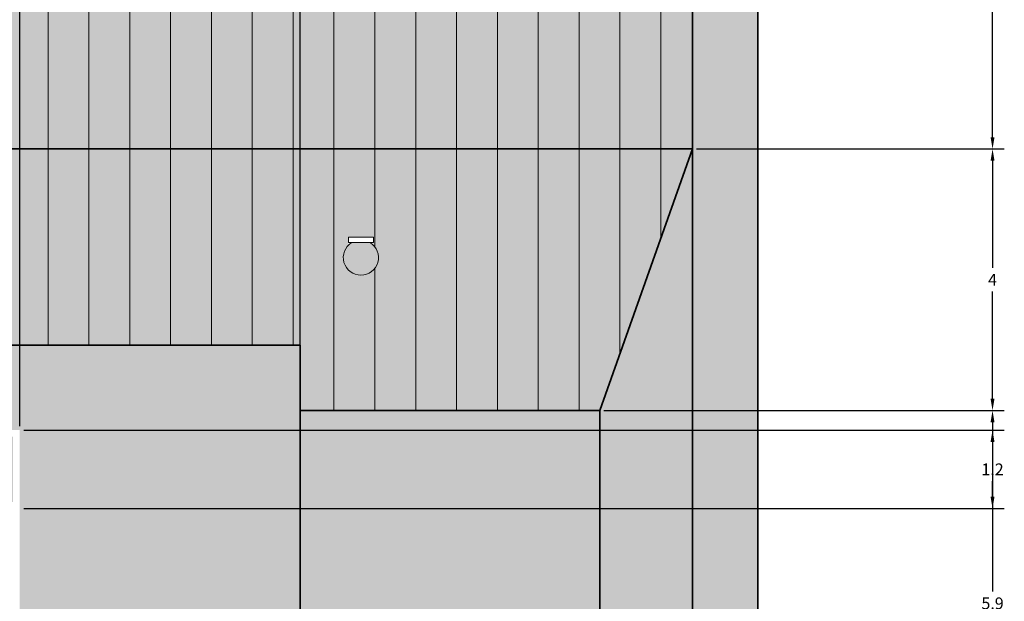
# Model space of a CAD drawing. Units: inches. Extents: x 18 to 59.8, y 2.7 to 81.2.
# Tile 9 of 9: x 44.6 to 59.6, y 54.5 to 63.4. Entities that reach past the tile are written whole.
import ezdxf

# ---------------------------------------------------------------- set-up
doc = ezdxf.new("R2010")
doc.units = ezdxf.units.IN
doc.header["$MEASUREMENT"] = 0
for name, color, linetype, lineweight in [('A-ANNO-DIMS', 2, 'Continuous', 18), ('A-ELEV', 7, 'Continuous', 35), ('A-ELEV-PATT', 8, 'Continuous', 13), ('E-LITE', 2, 'Continuous', 18)]:
    doc.layers.add(name, color=color, linetype=linetype, lineweight=lineweight)
doc.styles.get("Standard").update_dxf_attribs({"font": 'arial.ttf'})
doc.dimstyles.get("Standard").update_dxf_attribs({"dimtxt": 0.18, "dimasz": 0.18, "dimexe": 0.18, "dimexo": 0.0625, "dimgap": 0.09, "dimtad": 0, "dimtih": 1, "dimtoh": 1, "dimdec": 1, "dimzin": 0, "dimdsep": 46, "dimlunit": 3, "dimtxsty": 'Standard', "dimcen": 0.09, "dimadec": 0, "dimazin": 0, "dimtfac": 1, "dimtdec": 1, "dimtofl": 0, "dimtmove": 0, "dimatfit": 3, "dimfxl": 1, "dimtolj": 1, "dimtzin": 0, "dimarcsym": 0})

# ---------------------------------------------------------------- blocks, each defined once
blk = doc.blocks.new('LIGHT-CEILING-SPOT')
blk.add_lwpolyline([(0.0786613461026633, 0.4966935902599801), (0.4594351322230353, 0.4966935902599801), (0.4594351322230353, 0.5789100459995425), (0.0786613461026633, 0.5789100459995425)], close=True)
blk.add_arc((0.2690482391628493, 0.2688350374553394), 0.2689667806744183, 122.0956315451972, 57.90436845480281)
blk = doc.blocks.new('*D19')
at = {"layer": 'A-ANNO-DIMS', "color": 0, "lineweight": -2, "transparency": 16777216}
for p, q in [((53.50256100000002, 57.44074800000003), (59.62997100000006, 57.44074800000003)), ((59.44997100000005, 57.26074800000002), (59.44997100000005, 54.67265113778992)), ((59.44997100000005, 51.72074800000003), (59.44997100000005, 54.30884486221012)), ((53.42247100000003, 51.54074800000003), (59.62997100000006, 51.54074800000003))]:
    blk.add_line(p, q, dxfattribs=at)
at = {"layer": 'A-ANNO-DIMS', "color": 0, "transparency": 16777216}
for points in [[(59.41997100000005, 57.26074800000002), (59.47997100000005, 57.26074800000002), (59.44997100000005, 57.44074800000003)], [(59.41997100000005, 51.72074800000003), (59.47997100000005, 51.72074800000003), (59.44997100000005, 51.54074800000003)]]:
    blk.add_solid(points, dxfattribs=at)
at = {"layer": 'Defpoints', "color": 0, "transparency": 16777216}
for p in [(53.44006100000003, 57.44074800000003), (59.44997100000005, 57.44074800000003), (53.35997100000003, 51.54074800000003)]:
    blk.add_point(p, dxfattribs=at)
at = {"layer": 'A-ANNO-DIMS', "color": 0, "transparency": 16777216, "insert": (59.44997100000005, 54.49074799999999), "char_height": 0.18, "attachment_point": 5}
blk.add_mtext('\\A1;5.9', dxfattribs=at)
blk = doc.blocks.new('*D20')
at = {"layer": 'A-ANNO-DIMS', "color": 0, "lineweight": -2, "transparency": 16777216}
for p, q in [((54.92247100000003, 61.44074800000002), (59.62997100000006, 61.44074800000002)), ((59.44997100000005, 61.26074800000003), (59.44997100000005, 59.62074800000003)), ((59.44997100000005, 57.62074800000003), (59.44997100000005, 59.26074800000002)), ((53.50256100000002, 57.44074800000003), (59.62997100000006, 57.44074800000003))]:
    blk.add_line(p, q, dxfattribs=at)
at = {"layer": 'A-ANNO-DIMS', "color": 0, "transparency": 16777216}
for points in [[(59.41997100000005, 61.26074800000003), (59.47997100000005, 61.26074800000003), (59.44997100000005, 61.44074800000002)], [(59.41997100000005, 57.62074800000003), (59.47997100000005, 57.62074800000003), (59.44997100000005, 57.44074800000003)]]:
    blk.add_solid(points, dxfattribs=at)
at = {"layer": 'Defpoints', "color": 0, "transparency": 16777216}
for p in [(54.85997100000003, 61.44074800000002), (59.44997100000005, 61.44074800000002), (53.44006100000003, 57.44074800000003)]:
    blk.add_point(p, dxfattribs=at)
at = {"layer": 'A-ANNO-DIMS', "color": 0, "transparency": 16777216, "insert": (59.44997100000006, 59.44074799999999), "char_height": 0.18, "attachment_point": 5}
blk.add_mtext('\\A1;4', dxfattribs=at)
blk = doc.blocks.new('*D21')
at = {"layer": 'A-ANNO-DIMS', "color": 0, "lineweight": -2, "transparency": 16777216}
for p, q in [((54.92247100000003, 69.44074800000001), (59.62997100000006, 69.44074800000001)), ((59.44997100000005, 69.26074800000002), (59.44997100000005, 65.62265113778993)), ((59.44997100000005, 61.62074800000002), (59.44997100000005, 65.25884486221013)), ((54.92247100000003, 61.44074800000002), (59.62997100000006, 61.44074800000002))]:
    blk.add_line(p, q, dxfattribs=at)
at = {"layer": 'A-ANNO-DIMS', "color": 0, "transparency": 16777216}
for points in [[(59.41997100000005, 69.26074800000002), (59.47997100000005, 69.26074800000002), (59.44997100000005, 69.44074800000001)], [(59.41997100000005, 61.62074800000002), (59.47997100000005, 61.62074800000002), (59.44997100000005, 61.44074800000002)]]:
    blk.add_solid(points, dxfattribs=at)
at = {"layer": 'Defpoints', "color": 0, "transparency": 16777216}
for p in [(54.85997100000003, 69.44074800000001), (59.44997100000005, 69.44074800000001), (54.85997100000003, 61.44074800000002)]:
    blk.add_point(p, dxfattribs=at)
at = {"layer": 'A-ANNO-DIMS', "color": 0, "transparency": 16777216, "insert": (59.44997100000006, 65.440748), "char_height": 0.18, "attachment_point": 5}
blk.add_mtext('\\A1;8', dxfattribs=at)
blk = doc.blocks.new('*D51')
at = {"layer": 'A-ANNO-DIMS', "color": 0, "lineweight": -2, "transparency": 16777216}
for p, q in [((34.011642, 44.50324799999999), (34.011642, 81.210748)), ((48.859971, 43.503248), (48.859971, 81.210748)), ((34.191642, 81.03074799999999), (40.98046543587994, 81.03074799999999)), ((48.679971, 81.03074799999999), (41.89114756412005, 81.03074799999999))]:
    blk.add_line(p, q, dxfattribs=at)
at = {"layer": 'A-ANNO-DIMS', "color": 0, "transparency": 16777216}
for points in [[(34.191642, 81.060748), (34.191642, 81.00074799999999), (34.011642, 81.03074799999999)], [(48.679971, 81.060748), (48.679971, 81.00074799999999), (48.859971, 81.03074799999999)]]:
    blk.add_solid(points, dxfattribs=at)
at = {"layer": 'Defpoints', "color": 0, "transparency": 16777216}
for p in [(48.859971, 81.03074799999999), (34.011642, 44.440748), (48.859971, 43.440748)]:
    blk.add_point(p, dxfattribs=at)
at = {"layer": 'A-ANNO-DIMS', "color": 0, "transparency": 16777216, "insert": (41.43580649999999, 81.03074799999999), "char_height": 0.18, "attachment_point": 5}
blk.add_mtext('\\A1;14.848', dxfattribs=at)
blk = doc.blocks.new('*D62')
at = {"layer": 'A-ANNO-DIMS', "color": 0, "lineweight": -2, "transparency": 16777216}
for p, q in [((32.567078, 57.203248), (32.567078, 81.210748)), ((44.567078, 57.203248), (44.567078, 81.210748)), ((32.747078, 81.03074799999999), (38.35754866848568, 81.03074799999999)), ((44.387078, 81.03074799999999), (38.77660733151433, 81.03074799999999))]:
    blk.add_line(p, q, dxfattribs=at)
at = {"layer": 'A-ANNO-DIMS', "color": 0, "transparency": 16777216}
for points in [[(32.747078, 81.060748), (32.747078, 81.00074799999999), (32.567078, 81.03074799999999)], [(44.387078, 81.060748), (44.387078, 81.00074799999999), (44.567078, 81.03074799999999)]]:
    blk.add_solid(points, dxfattribs=at)
at = {"layer": 'Defpoints', "color": 0, "transparency": 16777216}
for p in [(44.567078, 81.03074799999999), (32.567078, 57.140748), (44.567078, 57.140748)]:
    blk.add_point(p, dxfattribs=at)
at = {"layer": 'A-ANNO-DIMS', "color": 0, "transparency": 16777216, "insert": (38.567078, 81.03074799999999), "char_height": 0.18, "attachment_point": 5}
blk.add_mtext('\\A1;12', dxfattribs=at)
blk = doc.blocks.new('*D63')
at = {"layer": 'A-ANNO-DIMS', "color": 0, "lineweight": -2, "transparency": 16777216}
for p, q in [((44.567078, 57.203248), (44.567078, 81.210748)), ((48.859971, 58.503248), (48.859971, 81.210748)), ((44.747078, 81.03074799999999), (46.31619844270123, 81.03074799999999)), ((48.679971, 81.03074799999999), (47.11085055729877, 81.03074799999999))]:
    blk.add_line(p, q, dxfattribs=at)
at = {"layer": 'A-ANNO-DIMS', "color": 0, "transparency": 16777216}
for points in [[(44.747078, 81.060748), (44.747078, 81.00074799999999), (44.567078, 81.03074799999999)], [(48.679971, 81.060748), (48.679971, 81.00074799999999), (48.859971, 81.03074799999999)]]:
    blk.add_solid(points, dxfattribs=at)
at = {"layer": 'Defpoints', "color": 0, "transparency": 16777216}
for p in [(48.859971, 81.03074799999999), (48.859971, 58.440748), (44.567078, 57.140748)]:
    blk.add_point(p, dxfattribs=at)
at = {"layer": 'A-ANNO-DIMS', "color": 0, "transparency": 16777216, "insert": (46.7135245, 81.03074799999999), "char_height": 0.18, "attachment_point": 5}
blk.add_mtext('\\A1;4.293', dxfattribs=at)
blk = doc.blocks.new('*D64')
at = {"layer": 'A-ANNO-DIMS', "color": 0, "lineweight": -2, "transparency": 16777216}
for p, q in [((44.62957800000001, 57.14074800000003), (59.62997100000006, 57.14074800000004)), ((59.44997100000005, 56.96074800000004), (59.44997100000005, 56.7211163492497)), ((59.44997100000005, 56.12074800000003), (59.44997100000005, 56.36037965075037)), ((44.62957800000001, 55.94074800000003), (59.62997100000006, 55.94074800000004))]:
    blk.add_line(p, q, dxfattribs=at)
at = {"layer": 'A-ANNO-DIMS', "color": 0, "transparency": 16777216}
for points in [[(59.41997100000005, 56.96074800000004), (59.47997100000005, 56.96074800000004), (59.44997100000005, 57.14074800000004)], [(59.41997100000005, 56.12074800000003), (59.47997100000005, 56.12074800000003), (59.44997100000005, 55.94074800000004)]]:
    blk.add_solid(points, dxfattribs=at)
at = {"layer": 'Defpoints', "color": 0, "transparency": 16777216}
for p in [(44.56707800000001, 57.14074800000003), (59.44997100000005, 57.14074800000004), (44.56707800000001, 55.94074800000003)]:
    blk.add_point(p, dxfattribs=at)
at = {"layer": 'A-ANNO-DIMS', "color": 0, "transparency": 16777216, "insert": (59.44997100000005, 56.540748), "char_height": 0.18, "attachment_point": 5}
blk.add_mtext('\\A1;1.2', dxfattribs=at)

msp = doc.modelspace()

# ---------------------------------------------------------------- hatches: boundary and pattern name
at = {"layer": 'A-ELEV-PATT'}
h = msp.add_hatch(color=256, dxfattribs=at)
h.set_gradient(color1=(255, 255, 255), color2=(199, 200, 202))
h.paths.add_polyline_path([(38.85997087182833, 75.45212783007513, 0.4125526599533602), (36.85997087192615, 77.44074750583997), (21.85997087182832, 77.44074750583995), (21.85997087182832, 22.44074750583995), (22.85997087182833, 22.44074750583995), (48.85997087182833, 22.44074750583996), (48.85997087182833, 30.92342676155402, 0.4074472928332927), (48.33023903111634, 31.44074750583995), (30.40609029701442, 31.44074750583996, -0.7603989452129261), (34.01164157247843, 44.44074750583996), (47.85997087182832, 44.44074750583995, -0.4142135623730951), (48.85997087182833, 43.44074750583994), (48.85997087182833, 48.44074750583995, 0.4142135623730955), (47.85997087182832, 49.44074750583995), (32.23382408177119, 49.44074750583993, -0.2243141867862321), (27.84111392101349, 52.84266085519661, -0.8480128940945467), (38.85997087182833, 61.44074750583993)])
h.paths.add_polyline_path([(55.85997087182832, 77.44074750583995), (54.85997087182832, 77.44074750583997), (54.85997087182832, 22.24074750583996), (55.85997087182832, 22.24074750583995)])
h.paths.add_polyline_path([(54.85997087182832, 51.54074750583995), (53.44006084017791, 51.54074750583996), (53.44006084017792, 29.64074750583996), (54.85997087182832, 29.64074750583996)])
h.paths.add_polyline_path([(54.85997087182832, 61.44074750583993), (53.44006084017791, 57.44074750583993), (53.44006084017791, 51.64074750583996), (54.85997087182832, 51.64074750583996)])
h.paths.add_polyline_path([(54.85997087182832, 29.44074750583995), (54.47100875861361, 29.44074750583995), (54.47100875861361, 22.24074750583996), (54.85997087182832, 22.24074750583996)])
h.paths.add_polyline_path([(55.57447446325177, 22.24074750583995), (54.85997087182832, 22.24074750583996), (54.57447446325178, 22.24074750583996), (53.93466996146642, 21.792542566958), (54.58769880335594, 21.54947740208223)])
h.paths.add_polyline_path([(54.59913950424823, 21.54521903603421), (53.94430429933965, 21.78895655088426), (53.94430429933965, 18.44074750583995), (54.59913950424823, 18.44074750583995)])
h.paths.add_polyline_path([(53.94430429933965, 21.78895655088427), (53.93466996146642, 21.792542566958), (53.58162006229036, 21.54521903603422), (53.58162006229036, 18.44074750583995), (53.94430429933965, 18.44074750583994)])
h.paths.add_polyline_path([(53.36475139777029, 20.69276091189374), (52.89555240690669, 21.06460517556268), (52.89555240690669, 18.44074750583995), (53.3647513977703, 18.44074750583994)])
h.paths.add_polyline_path([(52.89555240690669, 21.06460517556268), (50.57752474318004, 19.44074750583995), (50.57752474318004, 18.44074750583995), (52.89555240690669, 18.44074750583995)])
h.paths.add_polyline_path([(53.58162006229036, 21.54521903603423), (52.89555240690668, 21.06460517556268), (53.3647513977703, 20.69276091189373), (53.58162006229036, 20.84468482967704)])
h.paths.add_polyline_path([(26.81093959479239, 19.44074750583995), (24.96715419074249, 20.84074750583995), (24.96715419074249, 18.44074750583995), (26.81093959479239, 18.44074750583995)])
h.paths.add_polyline_path([(24.96715419074249, 20.84074750583995), (24.41645576890079, 20.84268308307895), (24.41645576890079, 18.44074750583994), (24.96715419074249, 18.44074750583994)])
h.paths.add_polyline_path([(24.41645576890079, 20.84268308307895), (24.41645576890079, 21.25889692219009), (24.05877847081848, 21.5304839605815), (24.03006070560372, 21.51834150822755), (24.03006070560372, 18.44074750583995), (24.41645576890079, 18.44074750583995)])
h.paths.add_polyline_path([(24.03006070560372, 21.51834150822755), (23.41645576890078, 21.2588969221901), (23.41645576890078, 18.44074750583996), (24.03006070560372, 18.44074750583995)])
h.paths.add_polyline_path([(24.03006070560372, 21.51834150822755), (24.05877847081849, 21.53048396058151), (23.12336878669258, 22.24074750583995), (22.12336878669259, 22.24074750583996), (23.41645576890079, 21.2588969221901)])
h.paths.add_polyline_path([(24.41645576890079, 21.2588969221901), (24.41645576890079, 20.84268308307896), (24.96715419074249, 20.84074750583994)])
h.paths.add_polyline_path([(47.85997087182832, 18.44074750583995), (29.85997087182832, 18.44074750583995), (29.85997087182832, 6.440747505839951), (30.85997087182832, 6.440747505839937), (30.85997087182832, 17.44074750583995), (38.85997087182833, 17.44074750583995), (46.85997087182832, 17.44074750583995), (46.85997087182832, 6.440747505839937), (47.85997087182832, 6.440747505839958)])
h.paths.add_polyline_path([(54.57559250001032, 15.2149800477124), (54.57559250001032, 6.440747505839944), (55.85997087182832, 6.440747505839951), (55.85997087182832, 18.44074750583995), (47.85997087182832, 18.44074750583995), (47.85997087182832, 6.440747505839944), (49.14824210254597, 6.440747505839944), (49.14824210254597, 15.2149800477124, -1)])
h = msp.add_hatch(color=256, dxfattribs=at)
h.paths.add_polyline_path([(27.84111392101356, 52.84266085519647, -0.7443789445921651), (36.85997087182832, 61.44074750583993), (38.85997087182833, 61.44074750583993, 0.8480128940945556)])
h.paths.add_polyline_path([(47.85997087182832, 44.44074750583995), (34.01164157247843, 44.44074750583996, 0.7603989452129407), (30.40609029701462, 31.44074750583983, -0.7376245609052545), (34.01164157247731, 43.44074750583994), (47.85997087182831, 43.44074750583994, -0.4142135623730951), (48.85997087182832, 42.44074750583995), (48.85997087182833, 43.44074750583994, 0.4142135623730951)])
h.paths.add_polyline_path([(54.57559250001032, 15.2149800477124), (54.57559250001032, 6.440747505839951), (55.85997087182832, 6.440747505839951), (55.85997087182832, 18.44074750583995), (47.85997087182832, 18.44074750583995), (47.85997087182832, 6.440747505839944), (49.14824210254597, 6.440747505839944), (49.14824210254597, 15.2149800477124, -1)])
h.paths.add_polyline_path([(47.85997087182832, 18.44074750583995), (29.85997087182832, 18.44074750583995), (29.85997087182832, 6.440747505839958), (30.85997087182832, 6.440747505839951), (30.85997087182832, 17.44074750583995), (38.85997087182833, 17.44074750583995), (46.85997087182832, 17.44074750583995), (46.85997087182832, 6.440747505839944), (47.85997087182832, 6.440747505839951)])
h.paths.add_polyline_path([(55.85997087182832, 77.44074750583995), (54.85997087182832, 77.44074750583997), (54.85997087182833, 22.24074750583995), (55.85997087182832, 22.24074750583995)])
h = msp.add_hatch(color=256, dxfattribs=at)
h.dxf.hatch_style = 1
h.paths.add_polyline_path([(54.85997087182832, 69.44074750583995), (38.85997087182833, 69.44074750583995), (38.85997087182833, 61.44074750583995), (54.85997087182832, 61.44074750583994)])
h.paths.add_polyline_path([(54.85997087182833, 61.44074750583994), (38.85997087182833, 61.44074750583995), (36.85997087182832, 61.44074750583993, 0.4434140223301819), (27.69861713021859, 58.44074750583995), (48.85997087182833, 58.44074750583995), (48.85997087182833, 57.44074750583994), (53.44006084017792, 57.44074750583995)])
h.paths.add_polyline_path([(37.49943513222304, 59.93991004599954), (37.49943513222304, 59.81982440572959, -2.410649922227508), (37.11866134610267, 59.81982440572959), (37.11866134610267, 59.93991004599954)], flags=16)
h.paths.add_polyline_path([(42.61253184194623, 59.80122867549901), (42.61253184194623, 59.92131431576897), (42.9933056280666, 59.92131431576897), (42.9933056280666, 59.80122867549901, -2.410649922227521)], flags=16)
h.paths.add_polyline_path([(49.59651616109447, 59.97095150496527), (49.59651616109447, 60.09103714523522), (49.97728994721485, 60.09103714523522), (49.97728994721485, 59.97095150496527, -2.410649922227521)], flags=16)
h.paths.add_polyline_path([(44.46707765301489, 57.04074750583994), (32.6670776530149, 57.04074750583994), (32.6670776530149, 56.04074750583993), (44.46707765301489, 56.04074750583993)])
h.paths.add_polyline_path([(47.85997087182831, 43.44074750583994), (46.85997087182832, 43.44074750583994), (34.0116415724774, 43.44074750583994, 0.2012982920418866), (29.34810857035394, 41.44074750583995), (47.85997087182831, 41.44074750583995, 1)])
h.paths.add_polyline_path([(36.55415719635351, 42.51454569609198), (36.55415719635351, 42.63463133636193), (36.93493098247388, 42.63463133636193), (36.93493098247388, 42.51454569609198, -2.410649922227513)], flags=16)
h.paths.add_polyline_path([(42.93899993637245, 42.54016758592221), (42.93899993637245, 42.66025322619216), (43.31977372249282, 42.66025322619216), (43.31977372249282, 42.54016758592221, -2.410649922227521)], flags=16)
h.paths.add_polyline_path([(54.47100875861361, 29.44074750583995), (48.85997087182833, 29.44074750583995), (48.85997087182833, 22.24074750583995), (54.47100875861361, 22.24074750583995)])
h.paths.add_polyline_path([(54.57447446325178, 22.24074750583996), (23.12336878669258, 22.24074750583996), (26.81093959479238, 19.44074750583996), (50.57752474318006, 19.44074750583996)])
h.paths.add_polyline_path([(54.57559250001032, 15.2149800477124, 1), (49.14824210254597, 15.2149800477124), (49.14824210254597, 6.440747505839958), (54.57559250001032, 6.440747505839965)])
h.paths.add_polyline_path([(49.83226884926398, 12.6020427608384), (49.83226884926398, 9.122455521673542), (49.66565363924473, 9.122455521673537), (49.66565363924473, 12.6020427608384)], flags=16)
h = msp.add_hatch(dxfattribs=at)
h.set_pattern_fill('ANSI31', color=256, scale=5, angle=45, style=0)
h.set_pattern_definition([(90, (0, 0), (-0.6250000000000001, 0), [])])
h.paths.add_polyline_path([(54.85997087182832, 69.44074750583995), (38.85997087182833, 69.44074750583995), (38.85997087182833, 61.44074750583995), (54.85997087182832, 61.44074750583994)])
h.paths.add_polyline_path([(54.85997087182833, 61.44074750583994), (38.85997087182833, 61.44074750583995), (36.85997087182832, 61.44074750583993, 0.4434140223301819), (27.69861713021859, 58.44074750583995), (48.85997087182833, 58.44074750583995), (48.85997087182833, 57.44074750583994), (53.44006084017792, 57.44074750583995)])
h.paths.add_polyline_path([(37.16613704638868, 59.85769359025997), (37.11866134610267, 59.85769359025997), (37.11866134610267, 59.93991004599954), (37.49943513222304, 59.93991004599954), (37.49943513222304, 59.85769359025997), (37.45195943193702, 59.85769359025997, -3.476462016968403)], flags=16)
h.paths.add_polyline_path([(42.66000754223224, 59.8390978600294), (42.61253184194623, 59.8390978600294), (42.61253184194623, 59.92131431576897), (42.9933056280666, 59.92131431576897), (42.9933056280666, 59.8390978600294), (42.94582992778058, 59.8390978600294, -3.47646201696846)], flags=16)
h.paths.add_polyline_path([(49.64399186138049, 60.00882068949565), (49.59651616109447, 60.00882068949565), (49.59651616109447, 60.09103714523522), (49.97728994721485, 60.09103714523522), (49.97728994721485, 60.00882068949565), (49.92981424692883, 60.00882068949565, -3.476462016968434)], flags=16)
h.paths.add_polyline_path([(44.46707765301489, 57.04074750583994), (32.6670776530149, 57.04074750583994), (32.6670776530149, 56.04074750583993), (44.46707765301489, 56.04074750583993)])
h.paths.add_polyline_path([(47.85997087182831, 43.44074750583994), (46.85997087182832, 43.44074750583994), (34.0116415724774, 43.44074750583994, 0.2012982920418866), (29.34810857035394, 41.44074750583995), (47.85997087182831, 41.44074750583995, 1)])
h.paths.add_polyline_path([(36.60163289663952, 42.55241488062237), (36.55415719635351, 42.55241488062236), (36.55415719635351, 42.63463133636193), (36.93493098247388, 42.63463133636193), (36.93493098247388, 42.55241488062236), (36.88745528218787, 42.55241488062236, -3.476462016968307)], flags=16)
h.paths.add_polyline_path([(42.98647563665846, 42.5780367704526), (42.93899993637245, 42.5780367704526), (42.93899993637245, 42.66025322619216), (43.31977372249282, 42.66025322619216), (43.31977372249282, 42.57803677045259), (43.2722980222068, 42.57803677045259, -3.476462016968351)], flags=16)
h.paths.add_polyline_path([(54.47100875861361, 29.44074750583995), (48.85997087182833, 29.44074750583995), (48.85997087182833, 22.24074750583995), (54.47100875861361, 22.24074750583994)])
h.paths.add_polyline_path([(54.57447446325179, 22.24074750583995), (23.12336878669258, 22.24074750583995), (26.81093959479238, 19.44074750583996), (50.57752474318005, 19.44074750583996)])
h.paths.add_polyline_path([(54.57559250001032, 15.2149800477124, 1), (49.14824210254597, 15.2149800477124), (49.14824210254597, 6.440747505839958), (54.57559250001032, 6.440747505839944)])
h.paths.add_polyline_path([(49.83226884926398, 9.122455521673542), (49.66565363924473, 9.122455521673537), (49.66565363924473, 12.60204276083839), (49.83226884926398, 12.6020427608384)], flags=16)
h = msp.add_hatch(color=256, dxfattribs=at)
h.paths.add_polyline_path([(36.88745528218787, 42.55241488062237), (36.60163289663952, 42.55241488062237, 3.476462016968434)])
h.paths.add_polyline_path([(43.2722980222068, 42.5780367704526), (42.98647563665846, 42.5780367704526, 3.476462016968434)])
h.paths.add_polyline_path([(37.45195943193702, 59.85769359025997), (37.16613704638868, 59.85769359025997, 3.476462016968438)])
h.paths.add_polyline_path([(42.94582992778058, 59.8390978600294), (42.66000754223224, 59.8390978600294, 3.476462016968421)])
h.paths.add_polyline_path([(49.92981424692883, 60.00882068949565), (49.64399186138049, 60.00882068949565, 3.47646201696846)])
edge = h.paths.add_edge_path()
edge.add_ellipse((29.03130355617049, 21.31074857073696), major_axis=(-0.2068459938827232, 0), ratio=0.4114480402009885, start_angle=0, end_angle=360)
edge = h.paths.add_edge_path()
edge.add_ellipse((32.59187600821468, 20.29631819013838), major_axis=(-0.2068459938827232, 0), ratio=0.4114480402009885, start_angle=0, end_angle=360)
edge = h.paths.add_edge_path()
edge.add_ellipse((35.50436209130413, 21.39076982130575), major_axis=(-0.2068459938827232, 0), ratio=0.4114480402009885, start_angle=0, end_angle=360)
edge = h.paths.add_edge_path()
edge.add_ellipse((39.38767712992086, 20.1968225557842), major_axis=(-0.2068459938827232, 0), ratio=0.4114480402009885, start_angle=0, end_angle=360)
edge = h.paths.add_edge_path()
edge.add_ellipse((43.2709921685377, 21.365896172764), major_axis=(-0.2068459938827232, 0), ratio=0.4114480402009885, start_angle=0, end_angle=360)
edge = h.paths.add_edge_path()
edge.add_ellipse((47.35345225115412, 20.14707456524252), major_axis=(-0.2068459938827232, 0), ratio=0.4114480402009885, start_angle=0, end_angle=360)
at = {"layer": 'A-ELEV-PATT', "transparency": 33554620}
h = msp.add_hatch(color=256, dxfattribs=at)
h.set_gradient(color1=(147, 149, 152))
edge = h.paths.add_edge_path()
edge.add_line((32.5670776530149, 55.94074750583994), (32.5670776530149, 57.14074750583994))
edge.add_line((32.5670776530149, 57.14074750583994), (44.5670776530149, 57.14074750583994))
edge.add_line((44.5670776530149, 57.14074750583994), (44.5670776530149, 55.94074750583994))
edge.add_line((44.5670776530149, 55.94074750583994), (44.56707765301487, 51.54074750583998))
edge.add_line((44.56707765301487, 51.54074750583998), (47.92075940082271, 51.54074750583998))
edge.add_spline(control_points=[(47.92075940082271, 51.54074750583998), (48.15238228194087, 51.51452682454292), (48.35972996747788, 51.37806491819363), (48.56707765301488, 51.24160301184435)], knot_values=[0, 0, 0, 0, 0.7121900809507601, 0.7121900809507601, 0.7121900809507601, 0.7121900809507601], degree=3, periodic=0)
edge.add_line((48.56707765301488, 51.24160301184435), (48.56707765301488, 49.14785428702649))
edge.add_arc((47.85997087182832, 48.44074750583995), 1, 5.739170477267294, 44.999999999999375, ccw=False)
edge.add_line((48.85495830893494, 48.54074750583996), (48.85997087182833, 48.54074750583996))
edge.add_line((48.85997087182833, 48.54074750583996), (48.85997087182833, 49.44074750583995))
edge.add_line((48.85997087182833, 49.44074750583995), (48.85997087182833, 58.44074750583995))
edge.add_line((48.85997087182833, 58.44074750583995), (27.6986171302186, 58.44074750583995))
edge.add_arc((33.63815495998532, 55.79107886226907), 6.503756879831279, 155.9580213816849, 220.80747886606)
edge.add_line((28.71539791616241, 51.54074750583994), (32.5670776530149, 51.54074750583994))
edge.add_line((32.5670776530149, 51.54074750583994), (32.5670776530149, 55.94074750583994))
edge = h.paths.add_edge_path()
edge.add_line((32.33023903111487, 40.44074750583996), (35.33023903111486, 40.44074750583996))
edge.add_line((35.33023903111486, 40.44074750583996), (38.33023903111485, 40.44074750583996))
edge.add_line((38.33023903111485, 40.44074750583996), (41.33023903111483, 40.44074750583996))
edge.add_line((41.33023903111483, 40.44074750583996), (44.33023903111482, 40.44074750583996))
edge.add_line((44.33023903111482, 40.44074750583996), (44.33023903111482, 33.83364072465343))
edge.add_line((44.33023903111482, 33.83364072465343), (47.68392077892264, 33.83364072465344))
edge.add_spline(control_points=[(47.68392077892267, 33.83364072465344), (47.91554366004082, 33.80742004335637), (48.12289134557783, 33.67095813700708), (48.33023903111483, 33.5344962306578)], knot_values=[0, 0, 0, 0, 0.7121900809507601, 0.7121900809507601, 0.7121900809507601, 0.7121900809507601], degree=3, periodic=0)
edge.add_line((48.33023903111483, 33.5344962306578), (48.33023903111483, 31.44074750583995))
edge.add_arc((48.3303844405005, 30.91101568508362), 0.5297318407134953, 1.3425044870115812, 90.01572747485528, ccw=False)
edge.add_line((48.85997087182833, 30.92342676155392), (48.85997087182833, 38.68456317332766))
edge.add_line((48.85997087182833, 38.68456317332766), (50.79297551695841, 38.68456317332766))
edge.add_line((50.79297551695841, 38.68456317332766), (50.79297551695841, 41.31595823441438))
edge.add_line((50.79297551695841, 41.31595823441438), (52.92696622669824, 41.31595823441438))
edge.add_line((52.92696622669824, 41.31595823441438), (52.92696622669824, 38.68456317332766))
edge.add_line((52.92696622669824, 38.68456317332766), (53.44006084017791, 38.68456317332766))
edge.add_line((53.44006084017791, 38.68456317332766), (53.44006084017791, 48.44074750583995))
edge.add_line((53.44006084017791, 48.44074750583995), (48.85997087182833, 48.44074750583995))
edge.add_line((48.85997087182833, 48.44074750583995), (48.85997087182832, 42.44074750583995))
edge.add_arc((47.85997087182831, 42.44074750583995), 1, -90, 0, ccw=False)
edge.add_line((47.85997087182831, 41.44074750583995), (29.34810857035394, 41.44074750583995))
edge.add_arc((34.06310194306089, 36.8836189221075), 6.557330511217327, 135.9754091201121, 207.7183105881144)
edge.add_line((28.25825772220566, 33.83364072465339), (32.33023903111487, 33.83364072465341))
edge.add_line((32.33023903111487, 33.83364072465341), (32.33023903111487, 40.44074750583996))
h.paths.add_polyline_path([(53.44006084017791, 57.44074750583995), (48.85997087182833, 57.44074750583994), (48.85997087182833, 51.64074750583996), (53.44006084017791, 51.64074750583996)])
h.paths.add_polyline_path([(29.56707765301488, 51.44074750583992), (28.80354322363853, 51.44074750583992, 0.040450980236505), (29.56707765301488, 50.71907894974708)], flags=17)
h.paths.add_polyline_path([(30.06707765301488, 51.44074750583992), (29.56707765301488, 51.44074750583992), (29.56707765301488, 50.71907894974708, 0.0237787432624053), (30.06707765301488, 50.35543166808938)], flags=17)
h.paths.add_polyline_path([(30.56707765301487, 51.44074750583993), (30.06707765301488, 51.44074750583992), (30.06707765301488, 50.35543166808938, 0.0223728768734236), (30.56707765301488, 50.05807461261393)], flags=17)
h.paths.add_polyline_path([(31.06707765301487, 51.44074750583993), (30.56707765301487, 51.44074750583993), (30.56707765301488, 50.05807461261393, 0.021345047641792), (31.06707765301488, 49.8171007041625)], flags=17)
h.paths.add_polyline_path([(31.56707765301487, 51.44074750583993), (31.06707765301487, 51.44074750583993), (31.06707765301488, 49.8171007041625, 0.0205857748313696), (31.56707765301488, 49.62589497689267)], flags=17)
h.paths.add_polyline_path([(32.06707765301488, 51.44074750583993), (31.56707765301487, 51.44074750583993), (31.56707765301488, 49.62589497689267, 0.0200299041308402), (32.06707765301488, 49.47993240164282)], flags=17)
h.paths.add_polyline_path([(32.5670776530149, 51.44074750583993), (32.06707765301488, 51.44074750583993), (32.06707765301488, 49.47993240164282, 0.0065845078177353), (32.23382408177119, 49.44074750583993), (32.5670776530149, 49.44074750583993)], flags=17)
h.paths.add_polyline_path([(45.06707765301486, 51.44074750583996), (44.56707765301487, 51.44074750583996), (44.56707765301487, 49.44074750583995), (45.06707765301488, 49.44074750583995)], flags=17)
h.paths.add_polyline_path([(45.56707765301488, 51.44074750583996), (45.06707765301486, 51.44074750583996), (45.06707765301488, 49.44074750583995), (45.56707765301488, 49.44074750583995)], flags=17)
h.paths.add_polyline_path([(46.06707765301488, 51.44074750583996), (45.56707765301488, 51.44074750583996), (45.56707765301488, 49.44074750583995), (46.06707765301488, 49.44074750583995)], flags=17)
h.paths.add_polyline_path([(46.56707765301487, 51.44074750583996), (46.06707765301488, 51.44074750583996), (46.06707765301488, 49.44074750583995), (46.56707765301487, 49.44074750583995)], flags=17)
h.paths.add_polyline_path([(47.06707765301487, 51.44074750583996), (46.56707765301487, 51.44074750583996), (46.56707765301487, 49.44074750583995), (47.06707765301487, 49.44074750583995)], flags=17)
h.paths.add_polyline_path([(47.56707765301487, 51.44074750583996), (47.06707765301487, 51.44074750583996), (47.06707765301487, 49.44074750583995), (47.56707765301488, 49.44074750583995)], flags=17)
edge = h.paths.add_edge_path(flags=17)
edge.add_spline(control_points=[(48.06707765301273, 51.41840713962396), (48.02172392661717, 51.43105064440995), (47.97524027779975, 51.4389035969284), (47.92733930740307, 51.44074750583996)], knot_values=[0.5701039528936005, 0.5701039528936005, 0.5701039528936005, 0.5701039528936005, 0.7151116034373463, 0.7151116034373463, 0.7151116034373463, 0.7151116034373644], degree=3, periodic=0)
edge.add_line((47.92733930740307, 51.44074750583996), (47.56707765301487, 51.44074750583996))
edge.add_line((47.56707765301487, 51.44074750583996), (47.56707765301488, 49.44074750583995))
edge.add_line((47.56707765301488, 49.44074750583995), (47.85997087182832, 49.44074750583995))
edge.add_arc((47.85997087182832, 48.44074750583995), 1, 78.04714410929728, 90, ccw=False)
edge.add_line((48.06707765301489, 49.41906584931846), (48.06707765301488, 51.41840713962341))
edge = h.paths.add_edge_path(flags=17)
edge.add_spline(control_points=[(48.56707765301488, 51.12118615879595), (48.40623273758901, 51.24494240176197), (48.24538782216315, 51.36869864472799), (48.06707765301273, 51.41840713962396)], knot_values=[0, 0, 0, 0, 0.5701039528936005, 0.5701039528936005, 0.5701039528936005, 0.5701039528936005], degree=3, periodic=0)
edge.add_line((48.06707765301488, 51.41840713962327), (48.06707765301489, 49.41906584931846))
edge.add_arc((47.85997087182832, 48.44074750583995), 1, 44.999999999999375, 78.04714410929728, ccw=False)
edge.add_line((48.56707765301488, 49.14785428702649), (48.56707765301488, 51.12118615879595))
h.paths.add_polyline_path([(49.35997087182833, 51.54074750583996), (48.85997087182833, 51.54074750583996), (48.85997087182833, 49.44074750583995), (48.85997087182833, 48.54074750583996), (49.35997087182833, 48.54074750583996)])
h.paths.add_polyline_path([(49.85997087182834, 51.54074750583996), (49.35997087182833, 51.54074750583996), (49.35997087182833, 48.54074750583996), (49.85997087182833, 48.54074750583996)])
h.paths.add_polyline_path([(50.35997087182834, 51.54074750583996), (49.85997087182834, 51.54074750583996), (49.85997087182833, 48.54074750583996), (50.35997087182833, 48.54074750583996)])
h.paths.add_polyline_path([(50.85997087182834, 51.54074750583996), (50.35997087182834, 51.54074750583996), (50.35997087182832, 48.54074750583996), (50.85997087182833, 48.54074750583996)])
h.paths.add_polyline_path([(51.35997087182833, 51.54074750583996), (50.85997087182834, 51.54074750583996), (50.85997087182833, 48.54074750583996), (51.35997087182833, 48.54074750583996)])
h.paths.add_polyline_path([(51.85997087182833, 51.54074750583996), (51.35997087182833, 51.54074750583996), (51.35997087182833, 48.54074750583995), (51.85997087182832, 48.54074750583995)])
h.paths.add_polyline_path([(52.35997087182834, 51.54074750583995), (51.85997087182833, 51.54074750583996), (51.85997087182832, 48.54074750583995), (52.35997087182834, 48.54074750583995)])
h.paths.add_polyline_path([(52.85997087182835, 51.54074750583995), (52.35997087182834, 51.54074750583995), (52.35997087182834, 48.54074750583995), (52.85997087182833, 48.54074750583995)])
h.paths.add_polyline_path([(53.35997087182834, 51.54074750583995), (52.85997087182835, 51.54074750583995), (52.85997087182833, 48.54074750583995), (53.35997087182834, 48.54074750583995)])
h.paths.add_polyline_path([(53.44006084017792, 38.68456317332766), (48.85997087182833, 38.68456317332766), (48.85997087182833, 30.92342676155392), (48.85997087182833, 29.64074750583995), (53.44006084017792, 29.64074750583994)])
h.paths.add_polyline_path([(28.83023903111483, 33.73364072465339), (28.31190895474052, 33.73364072465339, 0.0364451520675395), (28.83023903111484, 32.93194469741221)], flags=17)
h.paths.add_polyline_path([(29.33023903111483, 33.73364072465339), (28.83023903111483, 33.73364072465339), (28.83023903111484, 32.9319446974122, 0.0294200839082379), (29.33023903111484, 32.34505173740402)], flags=17)
h.paths.add_polyline_path([(29.83023903111483, 33.73364072465339), (29.33023903111483, 33.73364072465339), (29.33023903111484, 32.34505173740402, 0.0261691093073466), (29.83023903111483, 31.87548004603654)], flags=17)
h.paths.add_polyline_path([(30.33023903111483, 33.73364072465339), (29.83023903111483, 33.73364072465339), (29.83023903111483, 31.87548004603654, 0.0240262665661449), (30.33023903111483, 31.49248565404972)], flags=17)
h.paths.add_polyline_path([(30.83023903111483, 33.73364072465339), (30.33023903111483, 33.73364072465339), (30.33023903111483, 31.49248565404973, 0.0035005678246481), (30.40609029701443, 31.44074750583996), (30.83023903111484, 31.44074750583996)], flags=17)
h.paths.add_polyline_path([(31.33023903111483, 33.73364072465339), (30.83023903111483, 33.73364072465339), (30.83023903111484, 31.44074750583996), (31.33023903111483, 31.44074750583996)], flags=17)
h.paths.add_polyline_path([(31.83023903111483, 33.73364072465339), (31.33023903111483, 33.73364072465339), (31.33023903111483, 31.44074750583996), (31.83023903111483, 31.44074750583996)], flags=17)
h.paths.add_polyline_path([(32.33023903111487, 33.7336407246534), (31.83023903111483, 33.7336407246534), (31.83023903111483, 31.44074750583996), (32.33023903111487, 31.44074750583996)], flags=17)
h.paths.add_polyline_path([(44.83023903111482, 33.73364072465341), (44.33023903111482, 33.73364072465341), (44.33023903111482, 31.44074750583995), (44.83023903111483, 31.44074750583995)], flags=17)
h.paths.add_polyline_path([(45.33023903111483, 33.73364072465341), (44.83023903111482, 33.73364072465341), (44.83023903111483, 31.44074750583996), (45.33023903111483, 31.44074750583995)], flags=17)
h.paths.add_polyline_path([(45.83023903111483, 33.73364072465341), (45.33023903111483, 33.73364072465341), (45.33023903111483, 31.44074750583996), (45.83023903111483, 31.44074750583995)], flags=17)
h.paths.add_polyline_path([(46.33023903111483, 33.73364072465342), (45.83023903111483, 33.73364072465342), (45.83023903111483, 31.44074750583995), (46.33023903111482, 31.44074750583996)], flags=17)
h.paths.add_polyline_path([(46.83023903111482, 33.73364072465342), (46.33023903111483, 33.73364072465342), (46.33023903111482, 31.44074750583996), (46.83023903111482, 31.44074750583995)], flags=17)
h.paths.add_polyline_path([(47.33023903111482, 33.73364072465342), (46.83023903111482, 33.73364072465341), (46.83023903111482, 31.44074750583996), (47.33023903111484, 31.44074750583996)], flags=17)
edge = h.paths.add_edge_path(flags=16)
edge.add_spline(control_points=[(47.83023903111267, 33.71130035843739), (47.78488530471712, 33.7239438632234), (47.7384016558997, 33.73179681574185), (47.690500685503, 33.73364072465343)], knot_values=[0.5701039528936152, 0.5701039528936152, 0.5701039528936152, 0.5701039528936152, 0.7151116034373552, 0.7151116034373552, 0.7151116034373552, 0.7151116034373644], degree=3, periodic=0)
edge.add_line((47.69050068550314, 33.73364072465342), (47.33023903111482, 33.73364072465342))
edge.add_line((47.33023903111482, 33.73364072465342), (47.33023903111484, 31.44074750583995))
edge.add_line((47.33023903111484, 31.44074750583995), (47.83023903111484, 31.44074750583995))
edge.add_line((47.83023903111484, 31.44074750583995), (47.83023903111483, 33.71130035843684))
h.paths.add_polyline_path([(48.85997087182833, 38.68456317332766), (50.79297551695841, 38.68456317332766), (50.79297551695841, 41.31595823441438), (52.92696622669824, 41.31595823441438), (52.92696622669824, 38.68456317332766), (53.44006084017791, 38.68456317332766), (53.44006084017791, 48.44074750583995), (48.85997087182833, 48.44074750583995), (48.85997087182832, 42.44074750583995, -0.414213562373094), (47.85997087182831, 41.44074750583995), (29.34810857035394, 41.44074750583995, 0.3236799116418651), (28.25825772220566, 33.83364072465339), (32.33023903111487, 33.83364072465341), (32.33023903111487, 40.44074750583996), (35.33023903111486, 40.44074750583996), (38.33023903111485, 40.44074750583996), (41.33023903111483, 40.44074750583996), (44.33023903111482, 40.44074750583996), (44.33023903111482, 33.83364072465343), (28.25825772220566, 33.83364072465339, 0.0043266617348909), (28.31190895474052, 33.73364072465339), (28.83023903111483, 33.73364072465339), (29.33023903111483, 33.73364072465339), (29.83023903111483, 33.73364072465339), (30.33023903111483, 33.73364072465339), (30.83023903111483, 33.73364072465339), (31.33023903111483, 33.73364072465339), (31.83023903111483, 33.73364072465339), (32.33023903111487, 33.7336407246534), (47.33023903111482, 33.73364072465342), (47.33023903111484, 31.44074750583995), (47.83023903111484, 31.44074750583995), (48.33023903111591, 31.44074750583995, -0.4074472928335827), (48.85997087182833, 30.92342676155392)])
edge = h.paths.add_edge_path(flags=0)
edge.add_spline(control_points=[(47.83023903111267, 33.71130035843739), (47.78488530471713, 33.7239438632234), (47.73840165589972, 33.73179681574185), (47.69050068550303, 33.73364072465341)], knot_values=[0.5701039528936152, 0.5701039528936152, 0.5701039528936152, 0.5701039528936152, 0.7151116034373257, 0.7151116034373257, 0.7151116034373257, 0.7151116034373644], degree=3, periodic=0)
edge.add_line((47.69050068550293, 33.73364072465342), (47.33023903111482, 33.73364072465342))
edge.add_line((47.33023903111482, 33.73364072465342), (47.33023903111484, 31.44074750583995))
edge.add_line((47.33023903111484, 31.44074750583995), (47.83023903111484, 31.44074750583995))
edge.add_line((47.83023903111484, 31.44074750583995), (47.83023903111483, 33.71130035843687))

# ---------------------------------------------------------------- linework, layer by layer
at = {"layer": 'A-ELEV'}
for p, q in [((54.85997087182833, 22.24074750583995), (54.85997087182832, 77.44074750583995)), ((55.85997087182832, 77.44074750583994), (55.85997087182832, 22.24074750583995)), ((54.85997087182833, 61.44074750583994), (38.85997087182833, 61.44074750583995)), ((53.44006084017792, 57.44074750583995), (54.85997087182833, 61.44074750583994)), ((48.85997087182833, 58.44074750583995), (27.6986171302186, 58.44074750583995)), ((48.85997087182833, 42.44074750583995), (48.85997087182833, 58.44074750583994)), ((48.85997087182833, 57.44074750583994), (53.44006084017792, 57.44074750583995)), ((53.44006084017791, 57.44074750583996), (53.44006084017792, 29.64074750583995))]:
    msp.add_line(p, q, dxfattribs=at)

# ---------------------------------------------------------------- block references
at = {"layer": 'E-LITE'}
msp.add_blockref('LIGHT-CEILING-SPOT', (49.51785481499182, 59.51212709923567), dxfattribs=at)

# ---------------------------------------------------------------- dimensions: what is measured, and where the dimension line sits
at = {"layer": 'A-ANNO-DIMS'}
for base, p1, p2, override, picture, middle in [((44.567078, 81.03074799999999), (32.567078, 57.140748), (44.567078, 57.140748), {"dimdec": 0, "dimlfac": 1, "dimrnd": 0, "dimzin": 0, "dimdsep": 46, "dimlunit": 2}, '*D62', (38.567078, 81.03074799999999)), ((48.859971, 81.03074799999999), (34.011642, 44.440748), (48.859971, 43.440748), {"dimdec": 3, "dimlfac": 1, "dimrnd": 0, "dimzin": 0, "dimdsep": 46, "dimlunit": 2}, '*D51', (41.43580649999999, 81.03074799999999)), ((48.859971, 81.03074799999999), (44.567078, 57.140748), (48.859971, 58.440748), {"dimdec": 3, "dimlfac": 1, "dimrnd": 0, "dimzin": 0, "dimdsep": 46, "dimlunit": 2}, '*D63', (46.7135245, 81.03074799999999))]:
    dim = msp.add_linear_dim(base=base, p1=p1, p2=p2, dimstyle='Standard', override=override, dxfattribs=at)
    dim.commit()
    dim.dimension.update_dxf_attribs({"geometry": picture, "text_midpoint": middle})
for base, p1, p2, override, picture, middle in [((59.44997100000005, 69.44074800000001), (54.859971, 61.440748), (54.859971, 69.440748), {"dimdec": 0, "dimlfac": 1, "dimrnd": 0, "dimzin": 0, "dimdsep": 46, "dimlunit": 2}, '*D21', (59.44997100000006, 65.440748)), ((59.44997100000005, 61.44074800000002), (53.440061, 57.44074799999999), (54.859971, 61.440748), {"dimdec": 0, "dimlfac": 1, "dimrnd": 0, "dimzin": 0, "dimdsep": 46, "dimlunit": 2}, '*D20', (59.44997100000006, 59.44074799999999)), ((59.44997100000005, 57.44074800000003), (53.359971, 51.540748), (53.440061, 57.44074799999999), {"dimdec": 1, "dimlfac": 1, "dimrnd": 0, "dimzin": 0, "dimdsep": 46, "dimlunit": 2}, '*D19', (59.44997100000005, 54.49074799999999)), ((59.44997100000005, 57.14074800000004), (44.567078, 55.940748), (44.567078, 57.140748), {"dimdec": 1, "dimlfac": 1, "dimrnd": 0, "dimzin": 0, "dimdsep": 46, "dimlunit": 2}, '*D64', (59.44997100000005, 56.540748))]:
    dim = msp.add_linear_dim(base=base, p1=p1, p2=p2, angle=90, dimstyle='Standard', override=override, dxfattribs=at)
    dim.commit()
    dim.dimension.update_dxf_attribs({"geometry": picture, "text_midpoint": middle})

doc.saveas('drawing.dxf')
